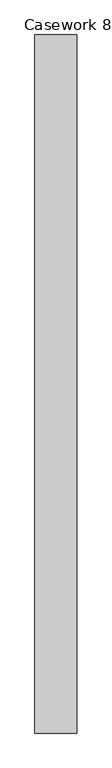
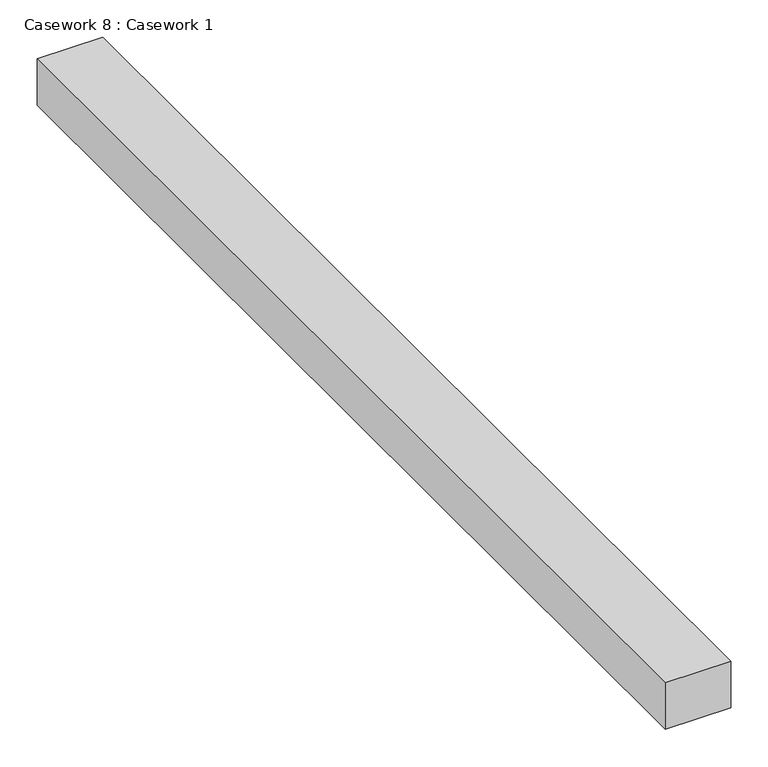
"""IFC4 building model written with IfcOpenShell, lengths in millimetres: furniture geometry, Casework 8 : Casework 1."""

from ifc_helpers import new_model, si_unit, frame, origin, place, context, project, spatial, polyline, outline, extrude, source, transform, mapped, element, save


def casework_8_casework_1_82254010(model_context):
    return source(origin(), model_context, "Body", "SweptSolid", [
        extrude(outline(polyline([(7528.9559589, 14787.9496924), (7528.9559589, 13098.8496924), (7427.3559589, 13098.8496924), (7427.3559589, 14787.9496924), (7528.9559589, 14787.9496924)])), frame((0.0, 0.0, 3581.4), z_axis=(0.0, 0.0, 1.0), x_axis=(1.0, 0.0, 0.0)), (0.0, 0.0, 1.0), 76.2),
    ])


if __name__ == "__main__":
    model = new_model("IFC4")
    model_context = context("Model", 3, world=origin())
    ifc_project = project(units=[si_unit("LENGTHUNIT", "METRE", prefix="MILLI")], contexts=[model_context])
    site = spatial("IfcSite", under=ifc_project)
    building = spatial("IfcBuilding", under=site)
    placement = place(None, origin())
    casework_8_casework_1_shape = casework_8_casework_1_82254010(model_context)
    element("IfcFurniture", 1, ObjectType="Casework 8 : Casework 1", at=placement, inside=building, context=model_context, shape_type="MappedRepresentation", body=[
        mapped(casework_8_casework_1_shape, transform((0.0, 0.0, 0.0), x_axis=(1.0, 0.0, 0.0), y_axis=(0.0, 1.0, 0.0), z_axis=(0.0, 0.0, 1.0))),
    ])
    save(model, "model.ifc")

# Revit data of these elements
# Element 1 (IfcFurniture, "Casework 8 : Casework 1")
#   Materials on its faces: "Clad - White"
# Materials
#   "Clad - White": class "Wood", colour RGB 242 242 238, transparency 0, Cost = 0
